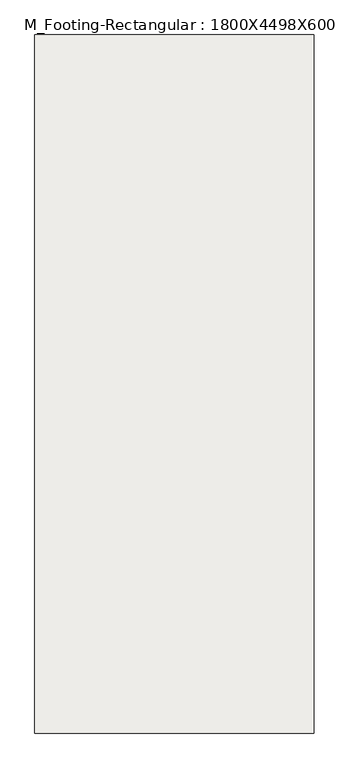
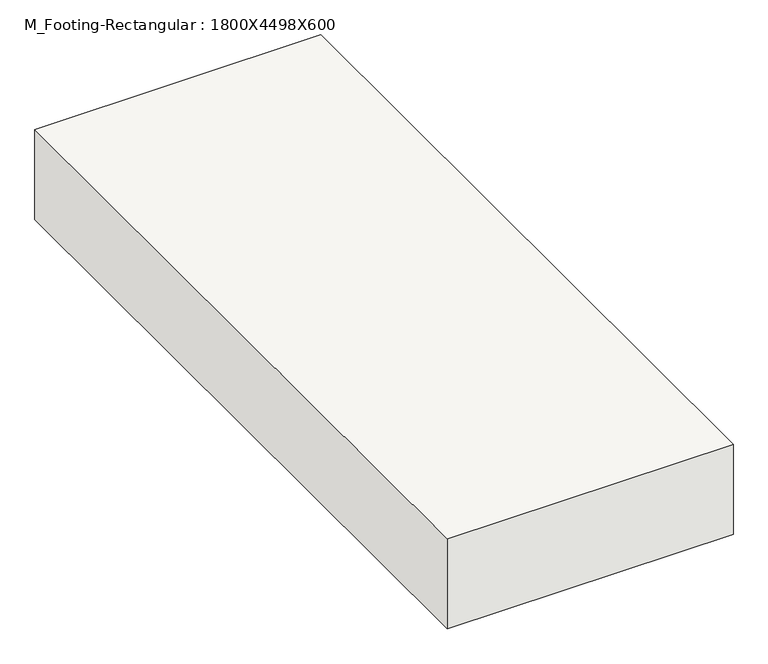
"""IFC4 building model written with IfcOpenShell, lengths in millimetres: slab geometry, M_Footing-Rectangular : 1800X4498X600."""

from ifc_helpers import new_model, si_unit, frame, origin, place, context, project, spatial, polyline, outline, extrude, source, transform, mapped, element, save


def m_footing_rectangular_1800x4498x600_2b6d0f7f(model_context):
    return source(origin(), model_context, "Body", "SweptSolid", [
        extrude(outline(polyline([(900.0, 2249.0), (900.0, -2249.0), (-900.0, -2249.0), (-900.0, 2249.0), (900.0, 2249.0)])), frame((0.0, 0.0, -600.0), z_axis=(0.0, 0.0, 1.0), x_axis=(1.0, 0.0, 0.0)), (0.0, 0.0, 1.0), 600.0),
    ])


if __name__ == "__main__":
    model = new_model("IFC4")
    model_context = context("Model", 3, world=origin())
    ifc_project = project(units=[si_unit("LENGTHUNIT", "METRE", prefix="MILLI")], contexts=[model_context])
    site = spatial("IfcSite", under=ifc_project)
    building = spatial("IfcBuilding", under=site)
    placement = place(None, origin())
    m_footing_rectangular_1800x4498x600_shape = m_footing_rectangular_1800x4498x600_2b6d0f7f(model_context)
    element("IfcSlab", 1, ObjectType="M_Footing-Rectangular : 1800X4498X600", at=placement, inside=building, context=model_context, shape_type="MappedRepresentation", body=[
        mapped(m_footing_rectangular_1800x4498x600_shape, transform((0.0, 0.0, 0.0), x_axis=(1.0, 0.0, 0.0), y_axis=(0.0, 1.0, 0.0), z_axis=(0.0, 0.0, 1.0))),
    ])
    save(model, "model.ifc")

# Revit data of these elements
# Type "M_Footing-Rectangular : 1800X4498X600"
#   Width = 1800 mm
#   Length = 4498 mm
#   Foundation Thickness = 600 mm
#   Structural Material [instance default] = Concrete, Cast-in-Place gray
#   Assembly Code = ""
# Element 1 (IfcSlab, "M_Footing-Rectangular : 1800X4498X600")
#   Structural Material = Concrete, Cast In Situ
#   Materials on its faces: "Concrete, Cast In Situ"
# Materials
#   "Concrete, Cast-in-Place gray": class "Concrete", colour RGB 192 192 192, transparency 0, Description = "Cast-in-place concrete", Cost = 0
#   "Concrete, Cast In Situ": class "Concrete", colour RGB 192 192 192, transparency 0, Description = "physical material", Cost = 0
